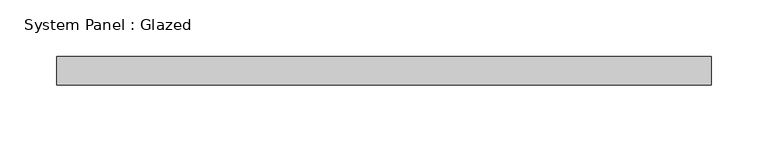
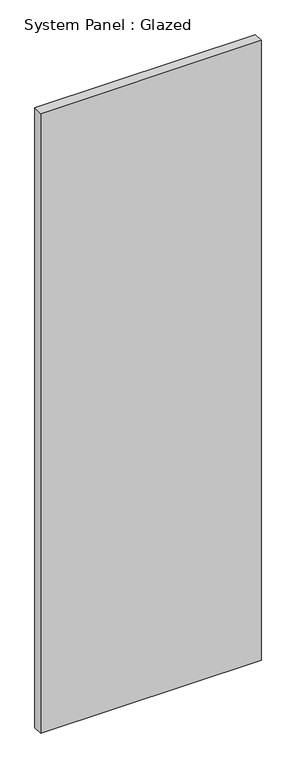
"""IFC4 building model written with IfcOpenShell, lengths in millimetres: plate geometry, System Panel : Glazed."""

from ifc_helpers import new_model, si_unit, origin, origin_with_axes, place, context, project, spatial, polyline, outline, extrude, source, transform, mapped, element, save


def system_panel_glazed_8fb17656(model_context):
    return source(origin(), model_context, "Body", "SweptSolid", [
        extrude(outline(polyline([(288.925, 19.05), (-288.925, 19.05), (-288.925, 44.45), (288.925, 44.45), (288.925, 19.05)])), origin_with_axes(), (0.0, 0.0, 1.0), 1716.0744962),
    ])


if __name__ == "__main__":
    model = new_model("IFC4")
    model_context = context("Model", 3, world=origin())
    ifc_project = project(units=[si_unit("LENGTHUNIT", "METRE", prefix="MILLI")], contexts=[model_context])
    site = spatial("IfcSite", under=ifc_project)
    building = spatial("IfcBuilding", under=site)
    placement = place(None, origin())
    system_panel_glazed_shape = system_panel_glazed_8fb17656(model_context)
    element("IfcPlate", 1, ObjectType="System Panel : Glazed", at=placement, inside=building, context=model_context, shape_type="MappedRepresentation", body=[
        mapped(system_panel_glazed_shape, transform((0.0, 0.0, 0.0), x_axis=(1.0, 0.0, 0.0), y_axis=(0.0, 1.0, 0.0), z_axis=(0.0, 0.0, 1.0))),
    ])
    save(model, "model.ifc")

# Revit data of these elements
# Type "System Panel : Glazed"
#   Construction Type Id = "GSP4R"
#   Analytic Construction = "1/8 in Pilkington single glazing"
#   Visual Light Transmittance = 0.9
#   Solar Heat Gain Coefficient = 0.86
#   Heat Transfer Coefficient (U) = 1.18115 BTU/(h·ft²·°F)
#   Define Thermal Properties by = 1
# Element 1 (IfcPlate, "System Panel : Glazed")
#   Materials on its faces: "Glass"
# Materials
#   "Glass": class "Glass", colour RGB 0 128 192, transparency 0.75, Description = "Soda Lime Glass", Cost = 0
